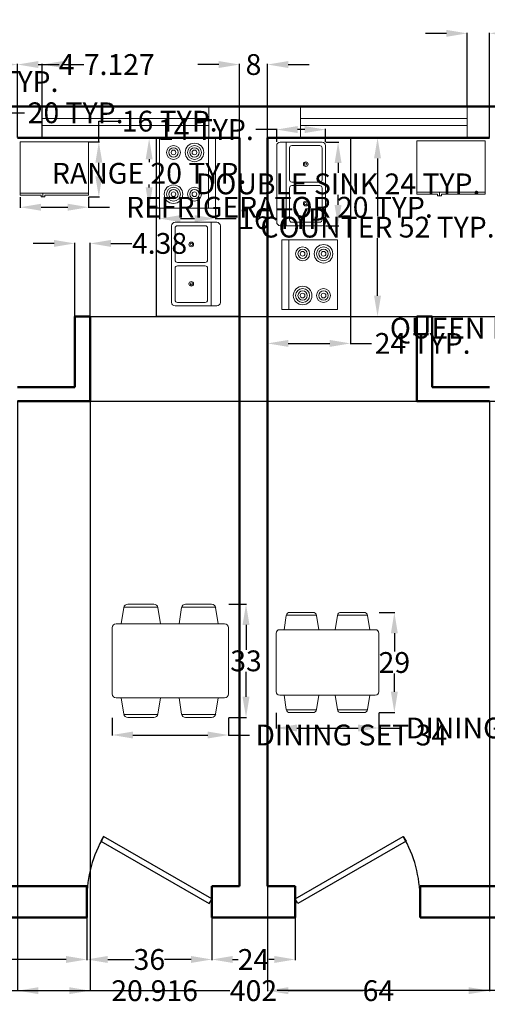
# Model space of a CAD drawing. Units: inches. Extents: x -22 to 471, y -231 to 53.
# Tile 2 of 3: x 143 to 277, y -231 to 53. Entities that reach past the tile are written whole.
import ezdxf

# ---------------------------------------------------------------- set-up
doc = ezdxf.new("R2010")
doc.units = ezdxf.units.IN
doc.header["$MEASUREMENT"] = 0
for name, color, linetype, lineweight in [('A-ANNO-DIMS', 2, 'Continuous', 18), ('A-DOOR', 3, 'Continuous', 25), ('A-EQPM', 9, 'Continuous', 18), ('A-FLOR-CASE', 32, 'Continuous', 25), ('A-FLOR-FIXT', 8, 'Continuous', 18), ('A-FURN', 8, 'Continuous', 18), ('A-GLAZ', 4, 'Continuous', 18), ('A-WALL', 7, 'Continuous', 50)]:
    doc.layers.add(name, color=color, linetype=linetype, lineweight=lineweight)
doc.styles.get("Standard").update_dxf_attribs({"font": 'arial.ttf'})
doc.dimstyles.get("Standard").update_dxf_attribs({"dimtxt": 6, "dimasz": 6, "dimexe": 0.18, "dimexo": 0.0625, "dimgap": 0.09, "dimtad": 0, "dimtih": 1, "dimtoh": 1, "dimdec": 0, "dimzin": 0, "dimdsep": 46, "dimlunit": 4, "dimtxsty": 'Standard', "dimcen": 0.09, "dimadec": 0, "dimazin": 0, "dimtfac": 1, "dimtdec": 0, "dimtofl": 0, "dimtmove": 0, "dimatfit": 3, "dimfxl": 1, "dimtolj": 1, "dimtzin": 0, "dimarcsym": 0})

# ---------------------------------------------------------------- blocks, each defined once
blk = doc.blocks.new('Range-Oven - 30 in top')
blk.add_line((0, -3), (30, -3))
blk.add_lwpolyline([(0, -24), (0, 0), (30, 0), (30, -24)], close=True)
for centre, radius in [((6, -9), 4), ((6, -9), 3), ((6, -9), 2), ((6, -9), 1), ((24, -9), 3), ((24, -9), 2), ((24, -9), 1), ((6, -18), 3), ((6, -18), 2), ((24, -18), 4), ((24, -18), 3), ((24, -18), 2), ((6, -18), 1), ((24, -18), 1)]:
    blk.add_circle(centre, radius)
blk = doc.blocks.new('Sink-double - 36 in top')
for p, q in [((-18, -4), (18, -4)), ((-0.75, -18.5), (-0.75, -6.5)), ((0.75, -6.5), (0.75, -18.5))]:
    blk.add_line(p, q)
for points in [[(-16.5, 0), (16.5, 0)], [(-18, -19.5), (-18, -1.5)], [(18, -1.5), (18, -19.5)], [(-16.5, -18.5), (-16.5, -6.5)], [(-15.5, -5.5), (-1.75, -5.5)], [(1.75, -5.5), (15.5, -5.5)], [(16.5, -6.5), (16.5, -18.5)], [(16.5, -21), (-16.5, -21)], [(-1.75, -19.5), (-15.5, -19.5)], [(15.5, -19.5), (1.75, -19.5)]]:
    blk.add_lwpolyline(points)
for centre, radius in [((-8.5, -12.5), 1), ((-8.5, -12.5), 0.5), ((8.5, -12.5), 1), ((8.5, -12.5), 0.5)]:
    blk.add_circle(centre, radius)
for centre, radius, start, end in [((-16.5, -1.5), 1.5, 90, 180), ((16.5, -1.5), 1.5, 0, 90), ((-15.5, -6.5), 1, 90, 180), ((-1.75, -6.5), 1, 0, 90), ((1.75, -6.5), 1, 90, 180), ((15.5, -6.5), 1, 0, 90), ((-16.5, -19.5), 1.5, 180, 270), ((-15.5, -18.5), 1, 180, 270), ((-1.75, -18.5), 1, 270, 0), ((1.75, -18.5), 1, 180, 270), ((15.5, -18.5), 1, 270, 0), ((16.5, -19.5), 1.5, 270, 0)]:
    blk.add_arc(centre, radius, start, end)
blk = doc.blocks.new('*U6')
for p, q in [((0, 0), (0, -6)), ((-40, 0), (-40, -6))]:
    blk.add_line(p, q)
blk.add_lwpolyline([(0, 0), (-34.64, 20), (-35.52, 18.48), (-0.88, -1.52)], close=True)
blk.add_arc((0, 0), 40, 150, 180)
blk = doc.blocks.new('*U5')
for p, q in [((0, 0), (0, -6)), ((40, 0), (40, -6))]:
    blk.add_line(p, q)
blk.add_lwpolyline([(0, 0), (34.64, 20), (35.52, 18.48), (0.87, -1.52)], close=True)
blk.add_arc((0, 0), 40, 0, 30)
blk = doc.blocks.new('Dining Set - 36 x 72 in.')
for p, q in [((-22.26, 25.81), (-23.48, 18)), ((-22.23, 26), (-5.76, 26)), ((-20.29, 27.5), (-7.71, 27.5)), ((-4.52, 18), (-5.74, 25.81)), ((5.74, 25.81), (4.52, 18)), ((5.77, 26), (22.24, 26)), ((7.71, 27.5), (20.29, 27.5)), ((23.48, 18), (22.26, 25.81)), ((-27.88, 16), (-27.88, -16)), ((26.5, 18), (-25.88, 18)), ((28.5, 16), (28.5, -16)), ((-25.88, -18), (26.5, -18)), ((-22.26, -25.81), (-23.48, -18)), ((-4.52, -18), (-5.74, -25.81)), ((5.74, -25.81), (4.52, -18)), ((23.48, -18), (22.26, -25.81)), ((-22.23, -26), (-5.76, -26)), ((-20.29, -27.5), (-7.71, -27.5)), ((5.77, -26), (22.24, -26)), ((7.71, -27.5), (20.29, -27.5))]:
    blk.add_line(p, q)
for centre, start, end in [((-20.29, 25.5), 90, 171.1198), ((-7.71, 25.5), 8.881, 90), ((7.71, 25.5), 90, 171.1198), ((20.29, 25.5), 8.881, 90), ((-25.88, 16), 90, 180), ((26.5, 16), 0, 90), ((-25.88, -16), 180, 270), ((26.5, -16), 270, 0), ((-20.29, -25.5), 188.8802, 270), ((-7.71, -25.5), 270, 351.1191), ((7.71, -25.5), 188.8802, 270), ((20.29, -25.5), 270, 351.1191)]:
    blk.add_arc(centre, 2, start, end)
blk = doc.blocks.new('Refrigerator-2 door - 36 in top')
for p, q in [((0, -26.999999), (36, -26.999999)), ((11, -27.999999), (11, -28.999999)), ((11, -28.999999), (13, -28.999999)), ((13, -28.999999), (13, -27.999999))]:
    blk.add_line(p, q)
blk.add_lwpolyline([(11, -27.999999), (0, -27.999999), (0, 0), (36, 0), (36, -27.999999), (13, -27.999999)])
blk = doc.blocks.new('WIN-48IN')
for p, q in [((0, 5.5), (48, 5.5)), ((0, 3.5), (48, 3.5))]:
    blk.add_line(p, q)
for points in [[(0, 0), (0, 9)], [(48, 9), (48, 0)]]:
    blk.add_lwpolyline(points)
blk = doc.blocks.new('KITCHEN-COUNTER')
for p in [(24, 51.62), (0, 0)]:
    blk.add_line(p, (24, 0))
blk = doc.blocks.new('*D17')
at = {"layer": 'A-ANNO-DIMS', "color": 0, "lineweight": -2, "transparency": 16777216}
for p, q in [((33.43, 28.07), (33.43, 35.39)), ((39.43, 35.21), (75.43, 35.21)), ((81.43, 28.07), (81.43, 35.39)), ((81.43, 35.21), (87.43, 35.21))]:
    blk.add_line(p, q, dxfattribs=at)
at = {"layer": 'A-ANNO-DIMS', "color": 0, "transparency": 16777216}
for points in [[(39.43, 36.21), (39.43, 34.21), (33.43, 35.21)], [(75.43, 36.21), (75.43, 34.21), (81.43, 35.21)]]:
    blk.add_solid(points, dxfattribs=at)
at = {"layer": 'Defpoints', "color": 0, "transparency": 16777216}
for p in [(81.43, 35.21), (33.43, 28.01), (81.43, 28.01)]:
    blk.add_point(p, dxfattribs=at)
at = {"layer": 'A-ANNO-DIMS', "color": 0, "transparency": 16777216, "insert": (121.8, 35.21), "char_height": 6, "attachment_point": 5}
blk.add_mtext('\\A1;WINDOW 48 TYP.', dxfattribs=at)
blk = doc.blocks.new('*D19')
at = {"layer": 'A-ANNO-DIMS', "color": 0, "lineweight": -2, "transparency": 16777216}
for p, q in [((318.71, 14.16), (303.56, 14.16)), ((303.74, 8.16), (303.74, -32.56)), ((303.74, -80.05), (303.74, -39.32)), ((318.71, -86.05), (303.56, -86.05))]:
    blk.add_line(p, q, dxfattribs=at)
at = {"layer": 'A-ANNO-DIMS', "color": 0, "transparency": 16777216}
for points in [[(302.74, 8.16), (304.74, 8.16), (303.74, 14.16)], [(302.74, -80.05), (304.74, -80.05), (303.74, -86.05)]]:
    blk.add_solid(points, dxfattribs=at)
at = {"layer": 'Defpoints', "color": 0, "transparency": 16777216}
for p in [(318.77, 14.16), (303.74, -86.05), (318.77, -86.05)]:
    blk.add_point(p, dxfattribs=at)
at = {"layer": 'A-ANNO-DIMS', "color": 0, "transparency": 16777216, "insert": (303.74, -35.94), "char_height": 6, "attachment_point": 5}
blk.add_mtext('\\A1;QUEEN BED GROUP 100 TYP.', dxfattribs=at)
blk = doc.blocks.new('*D21')
at = {"layer": 'A-ANNO-DIMS', "color": 0, "lineweight": -2, "transparency": 16777216}
for p, q in [((182.81, 18.77), (179.68, 18.77)), ((179.86, 12.77), (179.86, 11.91)), ((179.86, 4.68), (179.86, 5.53)), ((182.81, -1.32), (179.68, -1.32))]:
    blk.add_line(p, q, dxfattribs=at)
at = {"layer": 'A-ANNO-DIMS', "color": 0, "transparency": 16777216}
for points in [[(178.86, 12.77), (180.86, 12.77), (179.86, 18.77)], [(178.86, 4.68), (180.86, 4.68), (179.86, -1.32)]]:
    blk.add_solid(points, dxfattribs=at)
at = {"layer": 'Defpoints', "color": 0, "transparency": 16777216}
for p in [(182.87, 18.77), (179.86, -1.32), (182.87, -1.32)]:
    blk.add_point(p, dxfattribs=at)
at = {"layer": 'A-ANNO-DIMS', "color": 0, "transparency": 16777216, "insert": (179.86, 8.72), "char_height": 6, "attachment_point": 5}
blk.add_mtext('\\A1;RANGE 20 TYP.', dxfattribs=at)
blk = doc.blocks.new('*D22')
at = {"layer": 'A-ANNO-DIMS', "color": 0, "lineweight": -2, "transparency": 16777216}
for p, q in [((182.87, -1.39), (182.87, -4.52)), ((198.95, -1.39), (198.95, -4.52)), ((188.87, -4.34), (192.95, -4.34)), ((198.95, -4.34), (204.95, -4.34))]:
    blk.add_line(p, q, dxfattribs=at)
at = {"layer": 'A-ANNO-DIMS', "color": 0, "transparency": 16777216}
for points in [[(188.87, -3.34), (188.87, -5.34), (182.87, -4.34)], [(192.95, -3.34), (192.95, -5.34), (198.95, -4.34)]]:
    blk.add_solid(points, dxfattribs=at)
at = {"layer": 'Defpoints', "color": 0, "transparency": 16777216}
for p in [(182.87, -1.32), (198.95, -1.32), (198.95, -4.34)]:
    blk.add_point(p, dxfattribs=at)
at = {"layer": 'A-ANNO-DIMS', "color": 0, "transparency": 16777216, "insert": (219.36, -4.34), "char_height": 6, "attachment_point": 5}
blk.add_mtext('\\A1;16 TYP.', dxfattribs=at)
blk = doc.blocks.new('*D23')
at = {"layer": 'A-ANNO-DIMS', "color": 0, "lineweight": -2, "transparency": 16777216}
for p, q in [((230.76, 17.73), (234.49, 17.73)), ((234.31, 11.73), (234.31, 8.87)), ((234.31, -0.38), (234.31, 2.48)), ((230.76, -6.38), (234.49, -6.38))]:
    blk.add_line(p, q, dxfattribs=at)
at = {"layer": 'A-ANNO-DIMS', "color": 0, "transparency": 16777216}
for points in [[(233.31, 11.73), (235.31, 11.73), (234.31, 17.73)], [(233.31, -0.38), (235.31, -0.38), (234.31, -6.38)]]:
    blk.add_solid(points, dxfattribs=at)
at = {"layer": 'Defpoints', "color": 0, "transparency": 16777216}
for p in [(230.69, 17.73), (234.31, 17.73), (230.69, -6.38)]:
    blk.add_point(p, dxfattribs=at)
at = {"layer": 'A-ANNO-DIMS', "color": 0, "transparency": 16777216, "insert": (234.31, 5.68), "char_height": 6, "attachment_point": 5}
blk.add_mtext('\\A1;DOUBLE SINK 24 TYP.', dxfattribs=at)
blk = doc.blocks.new('*D24')
at = {"layer": 'A-ANNO-DIMS', "color": 0, "lineweight": -2, "transparency": 16777216}
for p, q in [((216.63, 21.35), (210.63, 21.35)), ((216.63, 17.79), (216.63, 21.53)), ((224.69, 21.35), (222.63, 21.35)), ((230.69, 17.79), (230.69, 21.53))]:
    blk.add_line(p, q, dxfattribs=at)
at = {"layer": 'A-ANNO-DIMS', "color": 0, "transparency": 16777216}
for points in [[(222.63, 22.35), (222.63, 20.35), (216.63, 21.35)], [(224.69, 22.35), (224.69, 20.35), (230.69, 21.35)]]:
    blk.add_solid(points, dxfattribs=at)
at = {"layer": 'Defpoints', "color": 0, "transparency": 16777216}
for p in [(216.63, 21.35), (216.63, 17.73), (230.69, 17.73)]:
    blk.add_point(p, dxfattribs=at)
at = {"layer": 'A-ANNO-DIMS', "color": 0, "transparency": 16777216, "insert": (196.22, 21.35), "char_height": 6, "attachment_point": 5}
blk.add_mtext('\\A1;14 TYP.', dxfattribs=at)
blk = doc.blocks.new('*D25')
at = {"layer": 'A-ANNO-DIMS', "color": 0, "lineweight": -2, "transparency": 16777216}
for p, q in [((169.19, -148.36), (169.19, -153.51)), ((202.74, -148.36), (202.74, -153.51)), ((175.19, -153.33), (196.74, -153.33)), ((202.74, -153.33), (208.74, -153.33))]:
    blk.add_line(p, q, dxfattribs=at)
at = {"layer": 'A-ANNO-DIMS', "color": 0, "transparency": 16777216}
for points in [[(175.19, -152.33), (175.19, -154.33), (169.19, -153.33)], [(196.74, -152.33), (196.74, -154.33), (202.74, -153.33)]]:
    blk.add_solid(points, dxfattribs=at)
at = {"layer": 'Defpoints', "color": 0, "transparency": 16777216}
for p in [(169.19, -148.3), (202.74, -148.3), (202.74, -153.33)]:
    blk.add_point(p, dxfattribs=at)
at = {"layer": 'A-ANNO-DIMS', "color": 0, "transparency": 16777216, "insert": (238.12, -153.33), "char_height": 6, "attachment_point": 5}
blk.add_mtext('\\A1;DINING SET 34', dxfattribs=at)
blk = doc.blocks.new('*D26')
at = {"layer": 'A-ANNO-DIMS', "color": 0, "lineweight": -2, "transparency": 16777216}
for p, q in [((202.81, -115.57), (207.96, -115.57)), ((207.78, -121.57), (207.78, -128.78)), ((207.78, -142.3), (207.78, -135.09)), ((202.81, -148.3), (207.96, -148.3))]:
    blk.add_line(p, q, dxfattribs=at)
at = {"layer": 'A-ANNO-DIMS', "color": 0, "transparency": 16777216}
for points in [[(206.78, -121.57), (208.78, -121.57), (207.78, -115.57)], [(206.78, -142.3), (208.78, -142.3), (207.78, -148.3)]]:
    blk.add_solid(points, dxfattribs=at)
at = {"layer": 'Defpoints', "color": 0, "transparency": 16777216}
for p in [(202.74, -115.57), (207.78, -115.57), (202.74, -148.3)]:
    blk.add_point(p, dxfattribs=at)
at = {"layer": 'A-ANNO-DIMS', "color": 0, "transparency": 16777216, "insert": (207.78, -131.94), "char_height": 6, "attachment_point": 5}
blk.add_mtext('\\A1;33', dxfattribs=at)
blk = doc.blocks.new('*D27')
at = {"layer": 'A-ANNO-DIMS', "color": 0, "lineweight": -2, "transparency": 16777216}
for p, q in [((216.44, -146.93), (216.44, -151.49)), ((246.08, -146.93), (246.08, -151.49)), ((222.44, -151.31), (240.08, -151.31)), ((246.08, -151.31), (252.08, -151.31))]:
    blk.add_line(p, q, dxfattribs=at)
at = {"layer": 'A-ANNO-DIMS', "color": 0, "transparency": 16777216}
for points in [[(222.44, -150.31), (222.44, -152.31), (216.44, -151.31)], [(240.08, -150.31), (240.08, -152.31), (246.08, -151.31)]]:
    blk.add_solid(points, dxfattribs=at)
at = {"layer": 'Defpoints', "color": 0, "transparency": 16777216}
for p in [(216.44, -146.86), (246.08, -146.86), (246.08, -151.31)]:
    blk.add_point(p, dxfattribs=at)
at = {"layer": 'A-ANNO-DIMS', "color": 0, "transparency": 16777216, "insert": (281.46, -151.31), "char_height": 6, "attachment_point": 5}
blk.add_mtext('\\A1;DINING SET 30', dxfattribs=at)
blk = doc.blocks.new('*D28')
at = {"layer": 'A-ANNO-DIMS', "color": 0, "lineweight": -2, "transparency": 16777216}
for p, q in [((246.14, -117.95), (250.71, -117.95)), ((250.53, -123.95), (250.53, -129.25)), ((250.53, -140.86), (250.53, -135.56)), ((246.14, -146.86), (250.71, -146.86))]:
    blk.add_line(p, q, dxfattribs=at)
at = {"layer": 'A-ANNO-DIMS', "color": 0, "transparency": 16777216}
for points in [[(249.53, -123.95), (251.53, -123.95), (250.53, -117.95)], [(249.53, -140.86), (251.53, -140.86), (250.53, -146.86)]]:
    blk.add_solid(points, dxfattribs=at)
at = {"layer": 'Defpoints', "color": 0, "transparency": 16777216}
for p in [(246.08, -117.95), (250.53, -117.95), (246.08, -146.86)]:
    blk.add_point(p, dxfattribs=at)
at = {"layer": 'A-ANNO-DIMS', "color": 0, "transparency": 16777216, "insert": (250.53, -132.41), "char_height": 6, "attachment_point": 5}
blk.add_mtext('\\A1;29', dxfattribs=at)
blk = doc.blocks.new('*D29')
at = {"layer": 'A-ANNO-DIMS', "color": 0, "lineweight": -2, "transparency": 16777216}
for p, q in [((142.7, 1.84), (142.7, -1.24)), ((162.42, 1.84), (162.42, -1.24)), ((148.7, -1.06), (156.42, -1.06)), ((162.42, -1.06), (168.42, -1.06))]:
    blk.add_line(p, q, dxfattribs=at)
at = {"layer": 'A-ANNO-DIMS', "color": 0, "transparency": 16777216}
for points in [[(148.7, -0.06), (148.7, -2.06), (142.7, -1.06)], [(156.42, -0.06), (156.42, -2.06), (162.42, -1.06)]]:
    blk.add_solid(points, dxfattribs=at)
at = {"layer": 'Defpoints', "color": 0, "transparency": 16777216}
for p in [(142.7, 1.9), (162.42, 1.9), (162.42, -1.06)]:
    blk.add_point(p, dxfattribs=at)
at = {"layer": 'A-ANNO-DIMS', "color": 0, "transparency": 16777216, "insert": (217.41, -1.06), "char_height": 6, "attachment_point": 5}
blk.add_mtext('\\A1;REFRIGERATOR 20 TYP.', dxfattribs=at)
blk = doc.blocks.new('*D30')
at = {"layer": 'A-ANNO-DIMS', "color": 0, "lineweight": -2, "transparency": 16777216}
for p, q in [((165.37, 17.78), (165.37, 23.78)), ((165.37, 23.78), (171.37, 23.78)), ((162.48, 17.78), (165.55, 17.78)), ((165.37, 7.9), (165.37, 11.78)), ((162.48, 1.9), (165.55, 1.9))]:
    blk.add_line(p, q, dxfattribs=at)
at = {"layer": 'A-ANNO-DIMS', "color": 0, "transparency": 16777216}
for points in [[(164.37, 11.78), (166.37, 11.78), (165.37, 17.78)], [(164.37, 7.9), (166.37, 7.9), (165.37, 1.9)]]:
    blk.add_solid(points, dxfattribs=at)
at = {"layer": 'Defpoints', "color": 0, "transparency": 16777216}
for p in [(162.42, 17.78), (165.37, 17.78), (162.42, 1.9)]:
    blk.add_point(p, dxfattribs=at)
at = {"layer": 'A-ANNO-DIMS', "color": 0, "transparency": 16777216, "insert": (185.78, 23.78), "char_height": 6, "attachment_point": 5}
blk.add_mtext('\\A1;16 TYP.', dxfattribs=at)
blk = doc.blocks.new('*D40')
at = {"layer": 'A-ANNO-DIMS', "color": 0, "lineweight": -2, "transparency": 16777216}
for p, q in [((117.9, 19.07), (117.9, 26.37)), ((123.9, 26.19), (131.93, 26.19)), ((137.93, 19.07), (137.93, 26.37)), ((137.93, 26.19), (143.93, 26.19))]:
    blk.add_line(p, q, dxfattribs=at)
at = {"layer": 'A-ANNO-DIMS', "color": 0, "transparency": 16777216}
for points in [[(123.9, 27.19), (123.9, 25.19), (117.9, 26.19)], [(131.93, 27.19), (131.93, 25.19), (137.93, 26.19)]]:
    blk.add_solid(points, dxfattribs=at)
at = {"layer": 'Defpoints', "color": 0, "transparency": 16777216}
for p in [(137.93, 26.19), (117.9, 19.01), (137.93, 19.01)]:
    blk.add_point(p, dxfattribs=at)
at = {"layer": 'A-ANNO-DIMS', "color": 0, "transparency": 16777216, "insert": (158.68, 26.19), "char_height": 6, "attachment_point": 5}
blk.add_mtext('\\A1;20 TYP.', dxfattribs=at)
blk = doc.blocks.new('*D41')
at = {"layer": 'A-ANNO-DIMS', "color": 0, "lineweight": -2, "transparency": 16777216}
for p, q in [((238, 19.01), (245.86, 19.01)), ((245.68, 13.01), (245.68, -3.6)), ((245.68, -26.6), (245.68, -9.99)), ((238, -32.6), (245.86, -32.6))]:
    blk.add_line(p, q, dxfattribs=at)
at = {"layer": 'A-ANNO-DIMS', "color": 0, "transparency": 16777216}
for points in [[(244.68, 13.01), (246.68, 13.01), (245.68, 19.01)], [(244.68, -26.6), (246.68, -26.6), (245.68, -32.6)]]:
    blk.add_solid(points, dxfattribs=at)
at = {"layer": 'Defpoints', "color": 0, "transparency": 16777216}
for p in [(237.93, 19.01), (245.68, 19.01), (237.93, -32.6)]:
    blk.add_point(p, dxfattribs=at)
at = {"layer": 'A-ANNO-DIMS', "color": 0, "transparency": 16777216, "insert": (245.68, -6.8), "char_height": 6, "attachment_point": 5}
blk.add_mtext('\\A1;COUNTER 52 TYP.', dxfattribs=at)
blk = doc.blocks.new('*D42')
at = {"layer": 'A-ANNO-DIMS', "color": 0, "lineweight": -2, "transparency": 16777216}
for p, q in [((213.93, -32.67), (213.93, -40.53)), ((237.93, -32.67), (237.93, -40.53)), ((219.93, -40.35), (231.93, -40.35)), ((237.93, -40.35), (243.93, -40.35))]:
    blk.add_line(p, q, dxfattribs=at)
at = {"layer": 'A-ANNO-DIMS', "color": 0, "transparency": 16777216}
for points in [[(219.93, -39.35), (219.93, -41.35), (213.93, -40.35)], [(231.93, -39.35), (231.93, -41.35), (237.93, -40.35)]]:
    blk.add_solid(points, dxfattribs=at)
at = {"layer": 'Defpoints', "color": 0, "transparency": 16777216}
for p in [(213.93, -32.6), (237.93, -32.6), (237.93, -40.35)]:
    blk.add_point(p, dxfattribs=at)
at = {"layer": 'A-ANNO-DIMS', "color": 0, "transparency": 16777216, "insert": (258.68, -40.35), "char_height": 6, "attachment_point": 5}
blk.add_mtext('\\A1;24 TYP.', dxfattribs=at)
blk = doc.blocks.new('*D43')
at = {"layer": 'A-ANNO-DIMS', "color": 0, "lineweight": -2, "transparency": 16777216}
for p, q in [((8.93, -206.05), (8.93, -227.27)), ((410.93, -206.05), (410.93, -227.27)), ((14.93, -227.09), (203.13, -227.09)), ((404.93, -227.09), (216.74, -227.09))]:
    blk.add_line(p, q, dxfattribs=at)
at = {"layer": 'A-ANNO-DIMS', "color": 0, "transparency": 16777216}
for points in [[(14.93, -226.09), (14.93, -228.09), (8.93, -227.09)], [(404.93, -226.09), (404.93, -228.09), (410.93, -227.09)]]:
    blk.add_solid(points, dxfattribs=at)
at = {"layer": 'Defpoints', "color": 0, "transparency": 16777216}
for p in [(8.93, -205.99), (410.93, -205.99), (410.93, -227.09)]:
    blk.add_point(p, dxfattribs=at)
at = {"layer": 'A-ANNO-DIMS', "color": 0, "transparency": 16777216, "insert": (209.93, -227.09), "char_height": 6, "attachment_point": 5}
blk.add_mtext('\\A1;402', dxfattribs=at)
blk = doc.blocks.new('*D46')
at = {"layer": 'A-ANNO-DIMS', "color": 0, "lineweight": -2, "transparency": 16777216}
for p, q in [((135.93, 40.11), (129.93, 40.11)), ((141.93, 19.07), (141.93, 40.29)), ((149.06, 19.07), (149.06, 40.29)), ((155.06, 40.11), (161.06, 40.11))]:
    blk.add_line(p, q, dxfattribs=at)
at = {"layer": 'A-ANNO-DIMS', "color": 0, "transparency": 16777216}
for points in [[(135.93, 41.11), (135.93, 39.11), (141.93, 40.11)], [(155.06, 41.11), (155.06, 39.11), (149.06, 40.11)]]:
    blk.add_solid(points, dxfattribs=at)
at = {"layer": 'Defpoints', "color": 0, "transparency": 16777216}
for p in [(149.06, 40.11), (141.93, 19.01), (149.06, 19.01)]:
    blk.add_point(p, dxfattribs=at)
at = {"layer": 'A-ANNO-DIMS', "color": 0, "transparency": 16777216, "insert": (171.25, 40.11), "char_height": 6, "attachment_point": 5}
blk.add_mtext('\\A1;7.127', dxfattribs=at)
blk = doc.blocks.new('*D47')
at = {"layer": 'A-ANNO-DIMS', "color": 0, "lineweight": -2, "transparency": 16777216}
for p, q in [((265.52, 49.11), (259.52, 49.11)), ((271.52, 28.07), (271.52, 49.29)), ((277.93, 19.07), (277.93, 49.29)), ((283.93, 49.11), (289.93, 49.11))]:
    blk.add_line(p, q, dxfattribs=at)
at = {"layer": 'A-ANNO-DIMS', "color": 0, "transparency": 16777216}
for points in [[(265.52, 50.11), (265.52, 48.11), (271.52, 49.11)], [(283.93, 50.11), (283.93, 48.11), (277.93, 49.11)]]:
    blk.add_solid(points, dxfattribs=at)
at = {"layer": 'Defpoints', "color": 0, "transparency": 16777216}
for p in [(277.93, 49.11), (271.52, 28.01), (277.93, 19.01)]:
    blk.add_point(p, dxfattribs=at)
at = {"layer": 'A-ANNO-DIMS', "color": 0, "transparency": 16777216, "insert": (300.16, 49.11), "char_height": 6, "attachment_point": 5}
blk.add_mtext('\\A1;6.416', dxfattribs=at)
blk = doc.blocks.new('*D49')
at = {"layer": 'A-ANNO-DIMS', "color": 0, "lineweight": -2, "transparency": 16777216}
for p, q in [((17.93, -197.05), (17.93, -218.27)), ((161.93, -197.05), (161.93, -218.27)), ((23.93, -218.09), (83.51, -218.09)), ((155.93, -218.09), (96.36, -218.09))]:
    blk.add_line(p, q, dxfattribs=at)
at = {"layer": 'A-ANNO-DIMS', "color": 0, "transparency": 16777216}
for points in [[(23.93, -217.09), (23.93, -219.09), (17.93, -218.09)], [(155.93, -217.09), (155.93, -219.09), (161.93, -218.09)]]:
    blk.add_solid(points, dxfattribs=at)
at = {"layer": 'Defpoints', "color": 0, "transparency": 16777216}
for p in [(17.93, -196.99), (161.93, -196.99), (17.93, -218.09)]:
    blk.add_point(p, dxfattribs=at)
at = {"layer": 'A-ANNO-DIMS', "color": 0, "transparency": 16777216, "insert": (89.93, -218.09), "char_height": 6, "attachment_point": 5}
blk.add_mtext('\\A1;144', dxfattribs=at)
blk = doc.blocks.new('*D50')
at = {"layer": 'A-ANNO-DIMS', "color": 0, "lineweight": -2, "transparency": 16777216}
for p, q in [((161.93, -197.05), (161.93, -218.27)), ((197.93, -197.05), (197.93, -218.27)), ((167.93, -218.09), (175.55, -218.09)), ((191.93, -218.09), (184.32, -218.09))]:
    blk.add_line(p, q, dxfattribs=at)
at = {"layer": 'A-ANNO-DIMS', "color": 0, "transparency": 16777216}
for points in [[(167.93, -217.09), (167.93, -219.09), (161.93, -218.09)], [(191.93, -217.09), (191.93, -219.09), (197.93, -218.09)]]:
    blk.add_solid(points, dxfattribs=at)
at = {"layer": 'Defpoints', "color": 0, "transparency": 16777216}
for p in [(161.93, -196.99), (197.93, -196.99), (161.93, -218.09)]:
    blk.add_point(p, dxfattribs=at)
at = {"layer": 'A-ANNO-DIMS', "color": 0, "transparency": 16777216, "insert": (179.93, -218.09), "char_height": 6, "attachment_point": 5}
blk.add_mtext('\\A1;36', dxfattribs=at)
blk = doc.blocks.new('*D51')
at = {"layer": 'A-ANNO-DIMS', "color": 0, "lineweight": -2, "transparency": 16777216}
for p, q in [((197.93, -197.05), (197.93, -218.27)), ((221.93, -197.05), (221.93, -218.27)), ((203.93, -218.09), (205.51, -218.09)), ((215.93, -218.09), (214.36, -218.09))]:
    blk.add_line(p, q, dxfattribs=at)
at = {"layer": 'A-ANNO-DIMS', "color": 0, "transparency": 16777216}
for points in [[(203.93, -217.09), (203.93, -219.09), (197.93, -218.09)], [(215.93, -217.09), (215.93, -219.09), (221.93, -218.09)]]:
    blk.add_solid(points, dxfattribs=at)
at = {"layer": 'Defpoints', "color": 0, "transparency": 16777216}
for p in [(197.93, -196.99), (221.93, -196.99), (197.93, -218.09)]:
    blk.add_point(p, dxfattribs=at)
at = {"layer": 'A-ANNO-DIMS', "color": 0, "transparency": 16777216, "insert": (209.93, -218.09), "char_height": 6, "attachment_point": 5}
blk.add_mtext('\\A1;24', dxfattribs=at)
blk = doc.blocks.new('*D54')
at = {"layer": 'A-ANNO-DIMS', "color": 0, "lineweight": -2, "transparency": 16777216}
for p, q in [((131.93, 40.11), (125.93, 40.11)), ((137.93, 19.07), (137.93, 40.29)), ((141.93, 19.07), (141.93, 40.29)), ((147.93, 40.11), (153.93, 40.11))]:
    blk.add_line(p, q, dxfattribs=at)
at = {"layer": 'A-ANNO-DIMS', "color": 0, "transparency": 16777216}
for points in [[(131.93, 41.11), (131.93, 39.11), (137.93, 40.11)], [(147.93, 41.11), (147.93, 39.11), (141.93, 40.11)]]:
    blk.add_solid(points, dxfattribs=at)
at = {"layer": 'Defpoints', "color": 0, "transparency": 16777216}
for p in [(141.93, 40.11), (137.93, 19.01), (141.93, 19.01)]:
    blk.add_point(p, dxfattribs=at)
at = {"layer": 'A-ANNO-DIMS', "color": 0, "transparency": 16777216, "insert": (156.1, 40.11), "char_height": 6, "attachment_point": 5}
blk.add_mtext('\\A1;4', dxfattribs=at)
blk = doc.blocks.new('*D55')
at = {"layer": 'A-ANNO-DIMS', "color": 0, "lineweight": -2, "transparency": 16777216}
for p, q in [((213.93, -32.67), (213.93, -227.27)), ((277.93, -57.05), (277.93, -227.27)), ((219.93, -227.09), (241.54, -227.09)), ((271.93, -227.09), (250.33, -227.09))]:
    blk.add_line(p, q, dxfattribs=at)
at = {"layer": 'A-ANNO-DIMS', "color": 0, "transparency": 16777216}
for points in [[(219.93, -226.09), (219.93, -228.09), (213.93, -227.09)], [(271.93, -226.09), (271.93, -228.09), (277.93, -227.09)]]:
    blk.add_solid(points, dxfattribs=at)
at = {"layer": 'Defpoints', "color": 0, "transparency": 16777216}
for p in [(213.93, -32.6), (277.93, -56.99), (277.93, -227.09)]:
    blk.add_point(p, dxfattribs=at)
at = {"layer": 'A-ANNO-DIMS', "color": 0, "transparency": 16777216, "insert": (245.93, -227.09), "char_height": 6, "attachment_point": 5}
blk.add_mtext('\\A1;64', dxfattribs=at)
blk = doc.blocks.new('*D56')
at = {"layer": 'A-ANNO-DIMS', "color": 0, "lineweight": -2, "transparency": 16777216}
for p, q in [((199.934447, 40.111163), (193.934447, 40.111163)), ((205.934447, 19.073663), (205.934447, 40.291163)), ((213.934447, 19.073663), (213.934447, 40.291163)), ((219.934447, 40.111163), (225.934447, 40.111163))]:
    blk.add_line(p, q, dxfattribs=at)
at = {"layer": 'A-ANNO-DIMS', "color": 0, "transparency": 16777216}
for points in [[(199.934447, 41.111163), (199.934447, 39.111163), (205.934447, 40.111163)], [(219.934447, 41.111163), (219.934447, 39.111163), (213.934447, 40.111163)]]:
    blk.add_solid(points, dxfattribs=at)
at = {"layer": 'Defpoints', "color": 0, "transparency": 16777216}
for p in [(213.934447, 40.111163), (205.934447, 19.011163), (213.934447, 19.011163)]:
    blk.add_point(p, dxfattribs=at)
at = {"layer": 'A-ANNO-DIMS', "color": 0, "transparency": 16777216, "insert": (209.934447, 40.111163), "char_height": 6, "attachment_point": 5}
blk.add_mtext('\\A1;8', dxfattribs=at)
blk = doc.blocks.new('*D62')
at = {"layer": 'A-ANNO-DIMS', "color": 0, "lineweight": -2, "transparency": 16777216}
for p, q in [((141.93, -57.05), (141.93, -227.27)), ((162.85, -57.05), (162.85, -227.27)), ((147.93, -227.09), (156.85, -227.09)), ((162.85, -227.09), (168.85, -227.09))]:
    blk.add_line(p, q, dxfattribs=at)
at = {"layer": 'A-ANNO-DIMS', "color": 0, "transparency": 16777216}
for points in [[(147.93, -226.09), (147.93, -228.09), (141.93, -227.09)], [(156.85, -226.09), (156.85, -228.09), (162.85, -227.09)]]:
    blk.add_solid(points, dxfattribs=at)
at = {"layer": 'Defpoints', "color": 0, "transparency": 16777216}
for p in [(141.93, -56.99), (162.85, -56.99), (162.85, -227.09)]:
    blk.add_point(p, dxfattribs=at)
at = {"layer": 'A-ANNO-DIMS', "color": 0, "transparency": 16777216, "insert": (181.44, -227.09), "char_height": 6, "attachment_point": 5}
blk.add_mtext('\\A1;20.916', dxfattribs=at)
blk = doc.blocks.new('*D63')
at = {"layer": 'A-ANNO-DIMS', "color": 0, "lineweight": -2, "transparency": 16777216}
for p, q in [((162.91, -32.6), (432.21, -32.6)), ((432.03, -38.6), (432.03, -41.64)), ((432.03, -50.99), (432.03, -47.95)), ((162.91, -56.99), (432.21, -56.99))]:
    blk.add_line(p, q, dxfattribs=at)
at = {"layer": 'A-ANNO-DIMS', "color": 0, "transparency": 16777216}
for points in [[(431.03, -38.6), (433.03, -38.6), (432.03, -32.6)], [(431.03, -50.99), (433.03, -50.99), (432.03, -56.99)]]:
    blk.add_solid(points, dxfattribs=at)
at = {"layer": 'Defpoints', "color": 0, "transparency": 16777216}
for p in [(162.85, -32.6), (432.03, -32.6), (162.85, -56.99)]:
    blk.add_point(p, dxfattribs=at)
at = {"layer": 'A-ANNO-DIMS', "color": 0, "transparency": 16777216, "insert": (432.03, -44.8), "char_height": 6, "attachment_point": 5}
blk.add_mtext('\\A1;24.385', dxfattribs=at)
blk = doc.blocks.new('*D65')
at = {"layer": 'A-ANNO-DIMS', "color": 0, "lineweight": -2, "transparency": 16777216}
for p, q in [((158.47, -32.54), (158.47, -11.32)), ((162.85, -32.54), (162.85, -11.32)), ((152.47, -11.5), (146.47, -11.5)), ((168.85, -11.5), (174.85, -11.5))]:
    blk.add_line(p, q, dxfattribs=at)
at = {"layer": 'A-ANNO-DIMS', "color": 0, "transparency": 16777216}
for points in [[(152.47, -10.5), (152.47, -12.5), (158.47, -11.5)], [(168.85, -10.5), (168.85, -12.5), (162.85, -11.5)]]:
    blk.add_solid(points, dxfattribs=at)
at = {"layer": 'Defpoints', "color": 0, "transparency": 16777216}
for p in [(162.85, -11.5), (158.47, -32.6), (162.85, -32.6)]:
    blk.add_point(p, dxfattribs=at)
at = {"layer": 'A-ANNO-DIMS', "color": 0, "transparency": 16777216, "insert": (182.86, -11.5), "char_height": 6, "attachment_point": 5}
blk.add_mtext('\\A1;4.38', dxfattribs=at)

msp = doc.modelspace()

# ---------------------------------------------------------------- linework, layer by layer
at = {"layer": 'A-EQPM'}
for p, q in [((149.2697, 1.898), (149.2697, 2.9934)), ((263.5374, 2.1849), (263.5374, 3.2804))]:
    msp.add_line(p, q, dxfattribs=at)
at = {"layer": 'A-WALL'}
for p, q in [((141.9344, 19.0112), (205.9344, 19.0112)), ((205.9344, 19.0112), (205.9344, -196.9888)), ((277.9344, 19.0112), (213.9344, 19.0112)), ((213.9344, 19.0112), (213.9344, -196.9888)), ((158.4725, -52.9888), (158.4725, -32.6035)), ((158.4725, -32.6035), (162.85, -32.6035)), ((162.85, -32.6035), (162.85, -56.9888)), ((261.3964, -32.6035), (257.0189, -32.6035)), ((257.0189, -32.6035), (257.0189, -56.9888)), ((261.3964, -52.9888), (261.3964, -32.6035)), ((141.9344, -52.9888), (158.4725, -52.9888)), ((277.9344, -52.9888), (261.3964, -52.9888)), ((141.9344, -56.9888), (162.85, -56.9888)), ((277.9344, -56.9888), (257.0189, -56.9888)), ((161.9344, -196.9888), (17.9344, -196.9888)), ((161.9344, -196.9888), (161.9344, -205.9888)), ((205.9344, -196.9888), (197.9344, -196.9888)), ((197.9344, -196.9888), (197.9344, -205.9888)), ((213.9344, -196.9888), (221.9344, -196.9888)), ((221.9344, -196.9888), (221.9344, -205.9888)), ((257.9344, -196.9888), (401.9344, -196.9888)), ((257.9344, -196.9888), (257.9344, -205.9888))]:
    msp.add_line(p, q, dxfattribs=at)
for points in [[(161.9344, -205.9888), (8.9344, -205.9888), (8.9344, 28.0112), (218.9344, 28.0112)], [(257.9344, -205.9888), (410.9344, -205.9888), (410.9344, 28.0112), (200.9344, 28.0112)], [(218.9344, -205.9888), (197.9344, -205.9888)], [(200.9344, -205.9888), (221.9344, -205.9888)]]:
    msp.add_lwpolyline(points, dxfattribs=at)

# ---------------------------------------------------------------- block references
at = {"layer": 'A-DOOR', "xscale": 0.9, "yscale": 0.9, "zscale": 0.9}
for name, p in [('*U6', (197.9344, -200.5888)), ('*U5', (221.9344, -200.5888))]:
    msp.add_blockref(name, p, dxfattribs=at)
at = {"layer": 'A-EQPM', "xscale": 0.5477313420588351, "yscale": 0.5477313420588351, "zscale": 0.5477313420588351}
for p in [(142.697, 17.7822), (256.9646, 18.0691)]:
    msp.add_blockref('Refrigerator-2 door - 36 in top', p, dxfattribs=at)
at = {"layer": 'A-EQPM', "xscale": 0.669754959773441, "yscale": 0.669754959773441, "zscale": 0.669754959773441}
for p, rotation in [((198.9455, 18.7677), 270), ((218.0673, -30.5598), 89.99999999999999)]:
    msp.add_blockref('Range-Oven - 30 in top', p, dxfattribs=dict(at, rotation=rotation))
at = {"layer": 'A-FLOR-CASE', "extrusion": (0, 0, -1), "zscale": -1}
msp.add_blockref('KITCHEN-COUNTER', (-205.9349, -32.604), dxfattribs=at)
at = {"layer": 'A-FLOR-CASE'}
msp.add_blockref('KITCHEN-COUNTER', (213.934, -32.604), dxfattribs=at)
at = {"layer": 'A-FLOR-FIXT', "xscale": 0.669754959773441, "yscale": 0.669754959773441, "zscale": 0.669754959773441}
for p, rotation in [((216.6278, 5.6768), 89.99999999999999), ((200.385, -17.4689), 270)]:
    msp.add_blockref('Sink-double - 36 in top', p, dxfattribs=dict(at, rotation=rotation))
at = {"layer": 'A-FURN'}
for p, xscale, yscale, zscale in [((185.7859, -131.9359), 0.5950381128668109, 0.5950381128668109, 0.5950381128668109), ((231.0978, -132.4069), 0.5256812652450878, 0.5256812652450878, 0.5256812652450878)]:
    msp.add_blockref('Dining Set - 36 x 72 in.', p, dxfattribs=dict(at, xscale=xscale, yscale=yscale, zscale=zscale))
at = {"layer": 'A-GLAZ'}
for p in [(149.061, 19.011), (223.5182, 19.011)]:
    msp.add_blockref('WIN-48IN', p, dxfattribs=at)

# ---------------------------------------------------------------- dimensions: what is measured, and where the dimension line sits
at = {"layer": 'A-ANNO-DIMS'}
for base, p1, p2, override, picture, middle in [((277.9344, 49.1112), (271.5183, 28.0112), (277.9344, 19.0112), {"dimdec": 3, "dimlfac": 1, "dimrnd": 0, "dimzin": 0, "dimdsep": 46, "dimlunit": 2}, '*D47', (300.1622, 49.1112)), ((141.9344, 40.1112), (137.9344, 19.0112), (141.9344, 19.0112), {"dimdec": 0, "dimlfac": 1, "dimrnd": 0, "dimzin": 0, "dimdsep": 46, "dimlunit": 2}, '*D54', (156.0995, 40.1112)), ((213.9344, 40.1112), (205.9344, 19.0112), (213.9344, 19.0112), {"dimdec": 0, "dimlfac": 1, "dimrnd": 0, "dimzin": 0, "dimdsep": 46, "dimlunit": 2}, '*D56', (209.9344, 40.1112)), ((162.85, -11.5035), (158.4725, -32.6035), (162.85, -32.6035), {"dimdec": 2, "dimlfac": 1, "dimrnd": 0, "dimzin": 0, "dimdsep": 46, "dimlunit": 2}, '*D65', (182.8595, -11.5035)), ((277.9344, -227.0888), (213.9344, -32.6035), (277.9344, -56.9888), {"dimdec": 0, "dimlfac": 1, "dimrnd": 0, "dimzin": 0, "dimdsep": 46, "dimlunit": 2}, '*D55', (245.9344, -227.0888)), ((162.85, -227.0888), (141.9344, -56.9888), (162.85, -56.9888), {"dimdec": 3, "dimlfac": 1, "dimrnd": 0, "dimzin": 0, "dimdsep": 46, "dimlunit": 2}, '*D62', (181.4434, -227.0888)), ((410.9344, -227.0888), (8.9344, -205.9888), (410.9344, -205.9888), {"dimdec": 0, "dimlfac": 1, "dimrnd": 0, "dimzin": 0, "dimdsep": 46, "dimlunit": 2}, '*D43', (209.9344, -227.0888))]:
    dim = msp.add_linear_dim(base=base, p1=p1, p2=p2, dimstyle='Standard', override=override, dxfattribs=at)
    dim.commit()
    dim.dimension.update_dxf_attribs({"geometry": picture, "text_midpoint": middle})
for base, p1, p2, text, picture, middle in [((81.4306, 35.2112), (33.4306, 28.0112), (81.4306, 28.0112), 'WINDOW <> TYP.', '*D17', (121.7996, 35.2112)), ((137.9344, 26.1896), (117.9021, 19.0112), (137.9344, 19.0112), '<> TYP.', '*D40', (158.6786, 26.1896)), ((162.4153, -1.0598), (142.697, 1.898), (162.4153, 1.898), 'REFRIGERATOR <> TYP.', '*D29', (217.4139, -1.0598)), ((198.9455, -4.3389), (182.8714, -1.325), (198.9455, -1.325), '<> TYP.', '*D22', (219.3561, -4.3389)), ((237.9344, -40.3457), (213.9344, -32.6035), (237.9344, -32.6035), '<> TYP.', '*D42', (258.6786, -40.3457)), ((246.08, -151.3091), (216.4404, -146.8631), (246.08, -146.8631), 'DINING SET <>', '*D27', (281.4558, -151.3091)), ((202.7448, -153.332), (169.1946, -148.2994), (202.7448, -148.2994), 'DINING SET <>', '*D25', (238.1186, -153.332))]:
    dim = msp.add_linear_dim(base=base, p1=p1, p2=p2, text=text, dimstyle='Standard', override={"dimdec": 0, "dimlfac": 1, "dimrnd": 0, "dimzin": 0, "dimdsep": 46, "dimlunit": 2}, dxfattribs=at)
    dim.commit()
    dim.dimension.update_dxf_attribs({"geometry": picture, "text_midpoint": middle})
for base, p1, p2, angle, override, picture, middle in [((149.0611, 40.1112), (141.9344, 19.0112), (149.0611, 19.0112), 0, {"dimdec": 3, "dimlfac": 1, "dimrnd": 0, "dimzin": 0, "dimdsep": 46, "dimlunit": 2}, '*D46', (171.25, 40.1112)), ((432.0344, -32.6035), (162.85, -56.9888), (162.85, -32.6035), 90, {"dimdec": 3, "dimlfac": 1, "dimrnd": 0, "dimzin": 0, "dimdsep": 46, "dimlunit": 2}, '*D63', (432.0344, -44.7962)), ((207.7774, -115.5723), (202.7448, -148.2994), (202.7448, -115.5723), 90, {"dimdec": 0, "dimlfac": 1, "dimrnd": 0, "dimzin": 0, "dimdsep": 46, "dimlunit": 2}, '*D26', (207.7774, -131.9359)), ((250.526, -117.9507), (246.08, -146.8631), (246.08, -117.9507), 90, {"dimdec": 0, "dimlfac": 1, "dimrnd": 0, "dimzin": 0, "dimdsep": 46, "dimlunit": 2}, '*D28', (250.526, -132.4069)), ((17.9344, -218.0888), (161.9344, -196.9888), (17.9344, -196.9888), 180, {"dimdec": 0, "dimlfac": 1, "dimrnd": 0, "dimzin": 0, "dimdsep": 46, "dimlunit": 2}, '*D49', (89.9344, -218.0888)), ((161.9344, -218.0888), (197.9344, -196.9888), (161.9344, -196.9888), 180, {"dimdec": 0, "dimlfac": 1, "dimrnd": 0, "dimzin": 0, "dimdsep": 46, "dimlunit": 2}, '*D50', (179.9344, -218.0888)), ((197.9344, -218.0888), (221.9344, -196.9888), (197.9344, -196.9888), 180, {"dimdec": 0, "dimlfac": 1, "dimrnd": 0, "dimzin": 0, "dimdsep": 46, "dimlunit": 2}, '*D51', (209.9344, -218.0888))]:
    dim = msp.add_linear_dim(base=base, p1=p1, p2=p2, angle=angle, dimstyle='Standard', override=override, dxfattribs=at)
    dim.commit()
    dim.dimension.update_dxf_attribs({"geometry": picture, "text_midpoint": middle})
for base, p1, p2, angle, text, picture, middle in [((165.373, 17.7822), (162.4153, 1.898), (162.4153, 17.7822), 90, '<> TYP.', '*D30', (185.7836, 23.7822)), ((216.6278, 21.3491), (230.6927, 17.7324), (216.6278, 17.7324), 180, '<> TYP.', '*D24', (196.2172, 21.3491)), ((234.3094, 17.7324), (230.6927, -6.3788), (230.6927, 17.7324), 90, 'DOUBLE SINK <> TYP.', '*D23', (234.3094, 5.6768)), ((179.8575, -1.325), (182.8714, 18.7677), (182.8714, -1.325), 270, 'RANGE <> TYP.', '*D21', (179.8575, 8.7214)), ((245.6766, 19.0112), (237.9344, -32.6035), (237.9344, 19.0112), 90, 'COUNTER <> TYP.', '*D41', (245.6766, -6.7962)), ((303.7424, -86.0462), (318.774, 14.1648), (318.774, -86.0462), 270, 'QUEEN BED GROUP <> TYP.', '*D19', (303.7424, -35.9407))]:
    dim = msp.add_linear_dim(base=base, p1=p1, p2=p2, angle=angle, text=text, dimstyle='Standard', override={"dimdec": 0, "dimlfac": 1, "dimrnd": 0, "dimzin": 0, "dimdsep": 46, "dimlunit": 2}, dxfattribs=at)
    dim.commit()
    dim.dimension.update_dxf_attribs({"geometry": picture, "text_midpoint": middle})

doc.saveas('drawing.dxf')
